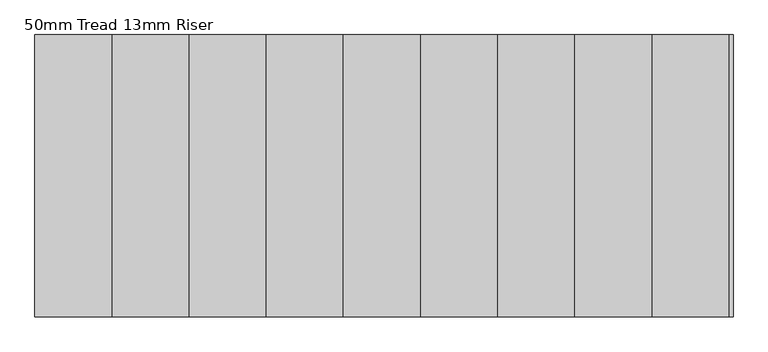
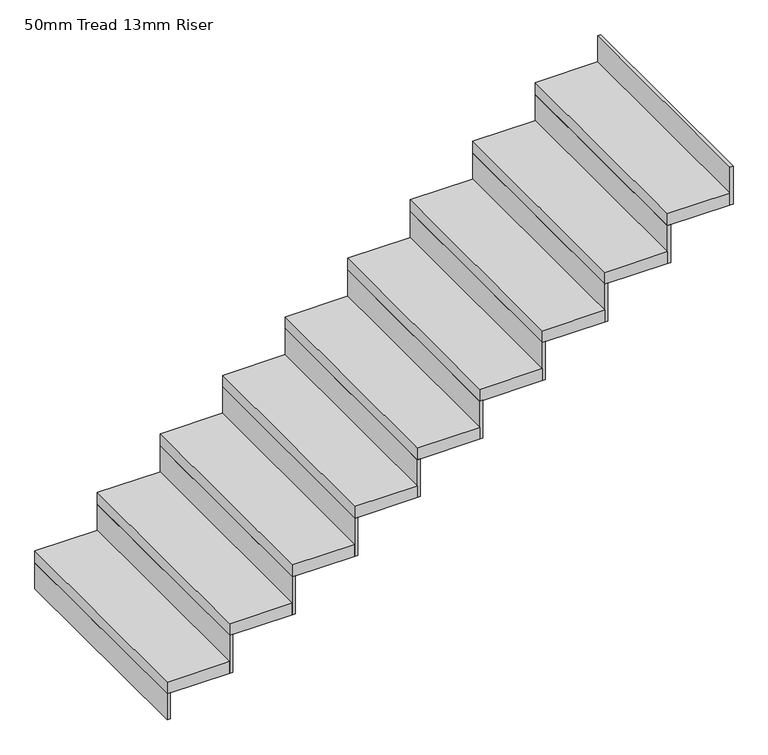
"""IFC4 building model written with IfcOpenShell, lengths in millimetres: stair flight geometry, 50mm Tread 13mm Riser."""

from ifc_helpers import new_model, si_unit, frame, origin, place, context, project, spatial, polyline, outline, extrude, source, transform, mapped, element, save


def stair_flight_50mm_tread_13mm_riser_06224c7e(model_context):
    return source(origin(), model_context, "Body", "SweptSolid", [
        extrude(outline(polyline([(-9782.9329612, -3037.6421603), (-9795.4329612, -3037.6421603), (-9795.4329612, -2123.2421603), (-9782.9329612, -2123.2421603), (-9782.9329612, -3037.6421603)])), frame((0.0, 0.0, 3200.4), z_axis=(0.0, 0.0, 1.0), x_axis=(1.0, 0.0, 0.0)), (0.0, 0.0, 1.0), 110.02),
        extrude(outline(polyline([(-9545.4329612, -2123.2421603), (-9545.4329612, -3037.6421603), (-9795.4329612, -3037.6421603), (-9795.4329612, -2123.2421603), (-9545.4329612, -2123.2421603)])), frame((0.0, 0.0, 3310.42), z_axis=(0.0, 0.0, 1.0), x_axis=(1.0, 0.0, 0.0)), (0.0, 0.0, 1.0), 50.0),
        extrude(outline(polyline([(-9532.9329612, -3037.6421603), (-9545.4329612, -3037.6421603), (-9545.4329612, -2123.2421603), (-9532.9329612, -2123.2421603), (-9532.9329612, -3037.6421603)])), frame((0.0, 0.0, 3310.42), z_axis=(0.0, 0.0, 1.0), x_axis=(1.0, 0.0, 0.0)), (0.0, 0.0, 1.0), 160.02),
        extrude(outline(polyline([(-9295.4329612, -2123.2421603), (-9295.4329612, -3037.6421603), (-9545.4329612, -3037.6421603), (-9545.4329612, -2123.2421603), (-9295.4329612, -2123.2421603)])), frame((0.0, 0.0, 3470.44), z_axis=(0.0, 0.0, 1.0), x_axis=(1.0, 0.0, 0.0)), (0.0, 0.0, 1.0), 50.0),
        extrude(outline(polyline([(-9282.9329612, -3037.6421603), (-9295.4329612, -3037.6421603), (-9295.4329612, -2123.2421603), (-9282.9329612, -2123.2421603), (-9282.9329612, -3037.6421603)])), frame((0.0, 0.0, 3470.44), z_axis=(0.0, 0.0, 1.0), x_axis=(1.0, 0.0, 0.0)), (0.0, 0.0, 1.0), 160.02),
        extrude(outline(polyline([(-9045.4329612, -2123.2421603), (-9045.4329612, -3037.6421603), (-9295.4329612, -3037.6421603), (-9295.4329612, -2123.2421603), (-9045.4329612, -2123.2421603)])), frame((0.0, 0.0, 3630.46), z_axis=(0.0, 0.0, 1.0), x_axis=(1.0, 0.0, 0.0)), (0.0, 0.0, 1.0), 50.0),
        extrude(outline(polyline([(-9032.9329612, -3037.6421603), (-9045.4329612, -3037.6421603), (-9045.4329612, -2123.2421603), (-9032.9329612, -2123.2421603), (-9032.9329612, -3037.6421603)])), frame((0.0, 0.0, 3630.46), z_axis=(0.0, 0.0, 1.0), x_axis=(1.0, 0.0, 0.0)), (0.0, 0.0, 1.0), 160.02),
        extrude(outline(polyline([(-8795.4329612, -2123.2421603), (-8795.4329612, -3037.6421603), (-9045.4329612, -3037.6421603), (-9045.4329612, -2123.2421603), (-8795.4329612, -2123.2421603)])), frame((0.0, 0.0, 3790.48), z_axis=(0.0, 0.0, 1.0), x_axis=(1.0, 0.0, 0.0)), (0.0, 0.0, 1.0), 50.0),
        extrude(outline(polyline([(-8782.9329612, -3037.6421603), (-8795.4329612, -3037.6421603), (-8795.4329612, -2123.2421603), (-8782.9329612, -2123.2421603), (-8782.9329612, -3037.6421603)])), frame((0.0, 0.0, 3790.48), z_axis=(0.0, 0.0, 1.0), x_axis=(1.0, 0.0, 0.0)), (0.0, 0.0, 1.0), 160.02),
        extrude(outline(polyline([(-8545.4329612, -2123.2421603), (-8545.4329612, -3037.6421603), (-8795.4329612, -3037.6421603), (-8795.4329612, -2123.2421603), (-8545.4329612, -2123.2421603)])), frame((0.0, 0.0, 3950.5), z_axis=(0.0, 0.0, 1.0), x_axis=(1.0, 0.0, 0.0)), (0.0, 0.0, 1.0), 50.0),
        extrude(outline(polyline([(-8532.9329612, -3037.6421603), (-8545.4329612, -3037.6421603), (-8545.4329612, -2123.2421603), (-8532.9329612, -2123.2421603), (-8532.9329612, -3037.6421603)])), frame((0.0, 0.0, 3950.5), z_axis=(0.0, 0.0, 1.0), x_axis=(1.0, 0.0, 0.0)), (0.0, 0.0, 1.0), 160.02),
        extrude(outline(polyline([(-8295.4329612, -2123.2421603), (-8295.4329612, -3037.6421603), (-8545.4329612, -3037.6421603), (-8545.4329612, -2123.2421603), (-8295.4329612, -2123.2421603)])), frame((0.0, 0.0, 4110.52), z_axis=(0.0, 0.0, 1.0), x_axis=(1.0, 0.0, 0.0)), (0.0, 0.0, 1.0), 50.0),
        extrude(outline(polyline([(-8282.9329612, -3037.6421603), (-8295.4329612, -3037.6421603), (-8295.4329612, -2123.2421603), (-8282.9329612, -2123.2421603), (-8282.9329612, -3037.6421603)])), frame((0.0, 0.0, 4110.52), z_axis=(0.0, 0.0, 1.0), x_axis=(1.0, 0.0, 0.0)), (0.0, 0.0, 1.0), 160.02),
        extrude(outline(polyline([(-8045.4329612, -2123.2421603), (-8045.4329612, -3037.6421603), (-8295.4329612, -3037.6421603), (-8295.4329612, -2123.2421603), (-8045.4329612, -2123.2421603)])), frame((0.0, 0.0, 4270.54), z_axis=(0.0, 0.0, 1.0), x_axis=(1.0, 0.0, 0.0)), (0.0, 0.0, 1.0), 50.0),
        extrude(outline(polyline([(-8032.9329612, -3037.6421603), (-8045.4329612, -3037.6421603), (-8045.4329612, -2123.2421603), (-8032.9329612, -2123.2421603), (-8032.9329612, -3037.6421603)])), frame((0.0, 0.0, 4270.54), z_axis=(0.0, 0.0, 1.0), x_axis=(1.0, 0.0, 0.0)), (0.0, 0.0, 1.0), 160.02),
        extrude(outline(polyline([(-7795.4329612, -2123.2421603), (-7795.4329612, -3037.6421603), (-8045.4329612, -3037.6421603), (-8045.4329612, -2123.2421603), (-7795.4329612, -2123.2421603)])), frame((0.0, 0.0, 4430.56), z_axis=(0.0, 0.0, 1.0), x_axis=(1.0, 0.0, 0.0)), (0.0, 0.0, 1.0), 50.0),
        extrude(outline(polyline([(-7782.9329612, -3037.6421603), (-7795.4329612, -3037.6421603), (-7795.4329612, -2123.2421603), (-7782.9329612, -2123.2421603), (-7782.9329612, -3037.6421603)])), frame((0.0, 0.0, 4430.56), z_axis=(0.0, 0.0, 1.0), x_axis=(1.0, 0.0, 0.0)), (0.0, 0.0, 1.0), 160.02),
        extrude(outline(polyline([(-7532.9329612, -3037.6421603), (-7545.4329612, -3037.6421603), (-7545.4329612, -2123.2421603), (-7532.9329612, -2123.2421603), (-7532.9329612, -3037.6421603)])), frame((0.0, 0.0, 4590.58), z_axis=(0.0, 0.0, 1.0), x_axis=(1.0, 0.0, 0.0)), (0.0, 0.0, 1.0), 160.02),
        extrude(outline(polyline([(-7545.4329612, -2123.2421603), (-7545.4329612, -3037.6421603), (-7795.4329612, -3037.6421603), (-7795.4329612, -2123.2421603), (-7545.4329612, -2123.2421603)])), frame((0.0, 0.0, 4590.58), z_axis=(0.0, 0.0, 1.0), x_axis=(1.0, 0.0, 0.0)), (0.0, 0.0, 1.0), 50.0),
    ])


if __name__ == "__main__":
    model = new_model("IFC4")
    model_context = context("Model", 3, world=origin())
    ifc_project = project(units=[si_unit("LENGTHUNIT", "METRE", prefix="MILLI")], contexts=[model_context])
    site = spatial("IfcSite", under=ifc_project)
    building = spatial("IfcBuilding", under=site)
    placement = place(None, origin())
    stair_flight_50mm_tread_13mm_riser_shape = stair_flight_50mm_tread_13mm_riser_06224c7e(model_context)
    element("IfcStairFlight", 1, ObjectType="50mm Tread 13mm Riser", at=placement, inside=building, context=model_context, shape_type="MappedRepresentation", body=[
        mapped(stair_flight_50mm_tread_13mm_riser_shape, transform((0.0, 0.0, 0.0), x_axis=(1.0, 0.0, 0.0), y_axis=(0.0, 1.0, 0.0), z_axis=(0.0, 0.0, 1.0))),
    ])
    save(model, "model.ifc")
